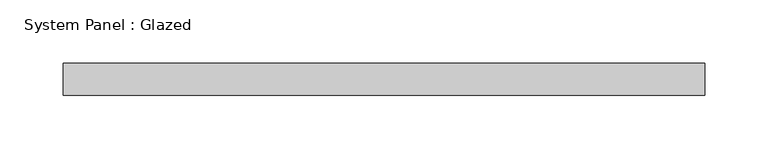
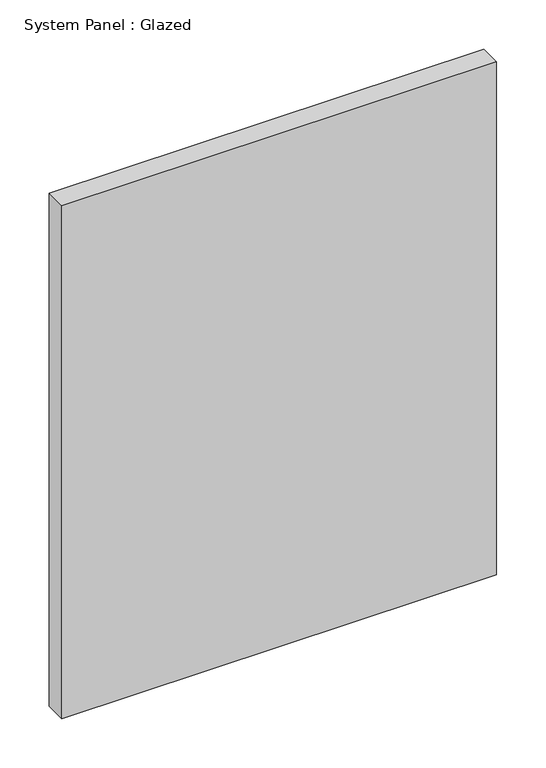
"""IFC4 building model written with IfcOpenShell, lengths in millimetres: plate geometry, System Panel : Glazed."""

from ifc_helpers import new_model, si_unit, origin, origin_with_axes, place, context, project, spatial, polyline, outline, extrude, source, transform, mapped, element, save


def system_panel_glazed_b26b014f(model_context):
    return source(origin(), model_context, "Body", "SweptSolid", [
        extrude(outline(polyline([(254.0, 19.05), (-254.0, 19.05), (-254.0, 44.45), (254.0, 44.45), (254.0, 19.05)])), origin_with_axes(), (0.0, 0.0, 1.0), 633.0738172),
    ])


if __name__ == "__main__":
    model = new_model("IFC4")
    model_context = context("Model", 3, world=origin())
    ifc_project = project(units=[si_unit("LENGTHUNIT", "METRE", prefix="MILLI")], contexts=[model_context])
    site = spatial("IfcSite", under=ifc_project)
    building = spatial("IfcBuilding", under=site)
    placement = place(None, origin())
    system_panel_glazed_shape = system_panel_glazed_b26b014f(model_context)
    element("IfcPlate", 1, ObjectType="System Panel : Glazed", at=placement, inside=building, context=model_context, shape_type="MappedRepresentation", body=[
        mapped(system_panel_glazed_shape, transform((0.0, 0.0, 0.0), x_axis=(1.0, 0.0, 0.0), y_axis=(0.0, 1.0, 0.0), z_axis=(0.0, 0.0, 1.0))),
    ])
    save(model, "model.ifc")

# Revit data of these elements
# Type "System Panel : Glazed"
#   Construction Type Id = "GSP4R"
#   Analytic Construction = "1/8 in Pilkington single glazing"
#   Visual Light Transmittance = 0.9
#   Solar Heat Gain Coefficient = 0.86
#   Heat Transfer Coefficient (U) = 1.18115 BTU/(h·ft²·°F)
#   Define Thermal Properties by = 1
# Element 1 (IfcPlate, "System Panel : Glazed")
#   Materials on its faces: "Glass"
# Materials
#   "Glass": class "Glass", colour RGB 0 128 192, transparency 0.75, Description = "Soda Lime Glass", Cost = 0
